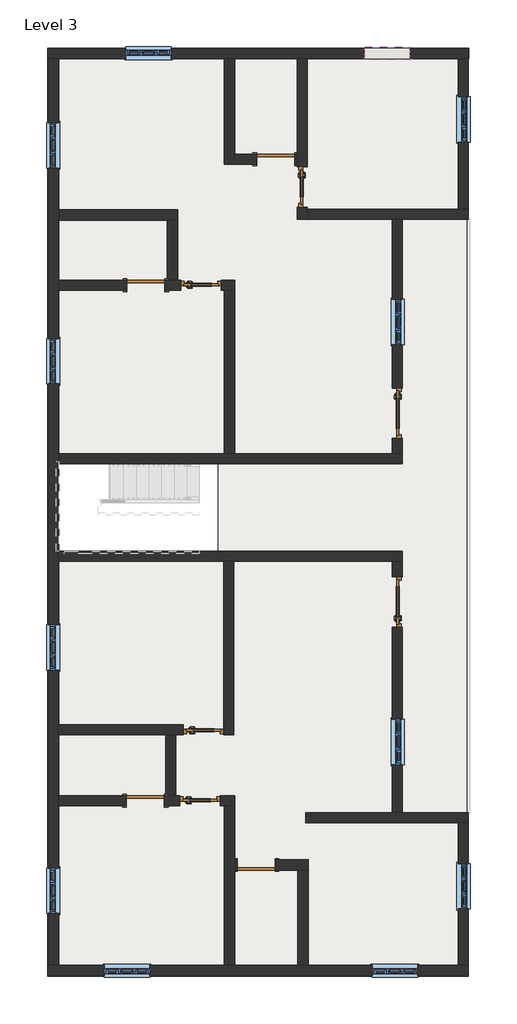
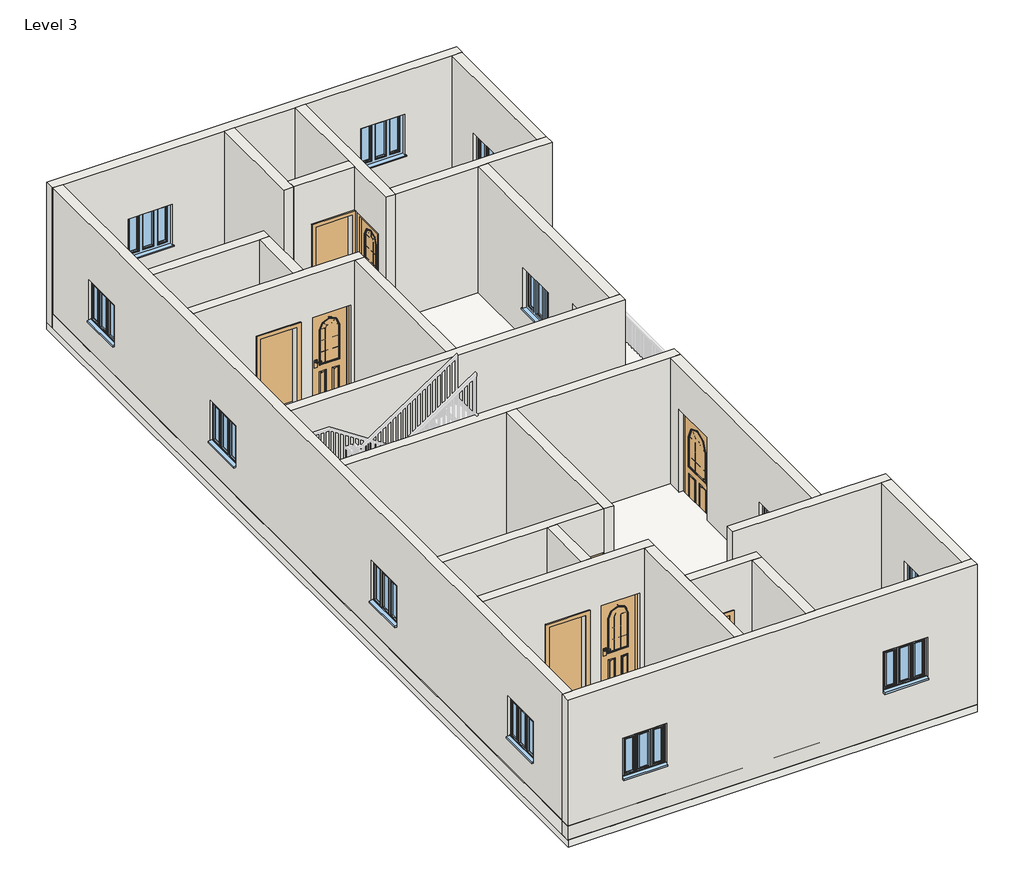
# One storey, part 1 of 3: 25 walls, 12 windows, 10 doors, 1 roof, 1 slab.
"""IFC4 building model written with IfcOpenShell, lengths in millimetres."""

from ifc_helpers import new_model, si_unit, frame, origin, place, context, project, spatial, polyline, outline, extrude, faceted_brep, transform, mapped, element, save
from components import doors_extsgl_w_glazing_bars_arched_1010x2110mm_bccdb1b2, doors_extsgl_w_glazing_bars_arched_1010x2110mm_5c897e1f, doors_extsgl_w_glazing_bars_arched_810x2110mm_57ea6d9e, doors_extsgl_w_glazing_bars_arched_810x2110mm_84a0a083, door_fadea3f2, windows_tpl_w_glazing_bars_910x910mm_9d987a72

model = new_model("IFC4")

# Units and contexts
model_context = context("Model", 3, world=origin())
ifc_project = project(units=[si_unit("LENGTHUNIT", "METRE", prefix="MILLI")], contexts=[model_context])

# Site, building, storey
site = spatial("IfcSite", under=ifc_project)
building = spatial("IfcBuilding", under=site)
storey = spatial("IfcBuildingStorey", under=building, Name="Level 3", Elevation=6096.0)

# Doors
placement = place(None, origin())
doors_extsgl_w_glazing_bars_arched_1010x2110mm_shape = doors_extsgl_w_glazing_bars_arched_1010x2110mm_bccdb1b2(model_context)
element("IfcDoor", 1, ObjectType="Doors_ExtSgl_w-Glazing_Bars_Arched : 1010x2110mm", at=placement, inside=storey, context=model_context, shape_type="MappedRepresentation", body=[
    mapped(doors_extsgl_w_glazing_bars_arched_1010x2110mm_shape, transform((1850.5605895, 2208.5797121, 6096.0), x_axis=(0.0, -1.0, 0.0), y_axis=(1.0, 0.0, 0.0), z_axis=(0.0, 0.0, 1.0))),
])
doors_extsgl_w_glazing_bars_arched_1010x2110mm_2_shape = doors_extsgl_w_glazing_bars_arched_1010x2110mm_5c897e1f(model_context)
element("IfcDoor", 2, ObjectType="Doors_ExtSgl_w-Glazing_Bars_Arched : 1010x2110mm", at=placement, inside=storey, context=model_context, shape_type="MappedRepresentation", body=[
    mapped(doors_extsgl_w_glazing_bars_arched_1010x2110mm_2_shape, transform((1850.5605895, -1576.0202879, 6096.0), x_axis=(0.0, 1.0, 0.0), y_axis=(-1.0, 0.0, 0.0), z_axis=(0.0, 0.0, 1.0))),
])
doors_extsgl_w_glazing_bars_arched_810x2110mm_shape = doors_extsgl_w_glazing_bars_arched_810x2110mm_57ea6d9e(model_context)
element("IfcDoor", 3, ObjectType="Doors_ExtSgl_w-Glazing_Bars_Arched : 810x2110mm", at=placement, inside=storey, context=model_context, shape_type="MappedRepresentation", body=[
    mapped(doors_extsgl_w_glazing_bars_arched_810x2110mm_shape, transform((-2086.4394105, 4773.9797121, 6096.0), x_axis=(1.0, 0.0, 0.0), y_axis=(0.0, 1.0, 0.0), z_axis=(0.0, 0.0, 1.0))),
])
element("IfcDoor", 4, ObjectType="Doors_ExtSgl_w-Glazing_Bars_Arched : 810x2110mm", at=placement, inside=storey, context=model_context, shape_type="MappedRepresentation", body=[
    mapped(doors_extsgl_w_glazing_bars_arched_810x2110mm_shape, transform((-2105.4894105, -5563.8202879, 6096.0), x_axis=(1.0, 0.0, 0.0), y_axis=(0.0, 1.0, 0.0), z_axis=(0.0, 0.0, 1.0))),
])
doors_extsgl_w_glazing_bars_arched_810x2110mm_2_shape = doors_extsgl_w_glazing_bars_arched_810x2110mm_84a0a083(model_context)
element("IfcDoor", 5, ObjectType="Doors_ExtSgl_w-Glazing_Bars_Arched : 810x2110mm", at=placement, inside=storey, context=model_context, shape_type="MappedRepresentation", body=[
    mapped(doors_extsgl_w_glazing_bars_arched_810x2110mm_2_shape, transform((-2035.6394105, -4141.4202879, 6096.0), x_axis=(1.0, 0.0, 0.0), y_axis=(0.0, 1.0, 0.0), z_axis=(0.0, 0.0, 1.0))),
])
element("IfcDoor", 6, ObjectType="Doors_ExtSgl_w-Glazing_Bars_Arched : 810x2110mm", at=placement, inside=storey, context=model_context, shape_type="MappedRepresentation", body=[
    mapped(doors_extsgl_w_glazing_bars_arched_810x2110mm_2_shape, transform((-54.4394105, 6748.5640518, 6096.0), x_axis=(0.0, -1.0, 0.0), y_axis=(1.0, 0.0, 0.0), z_axis=(0.0, 0.0, 1.0))),
])
door_shape = door_fadea3f2(model_context)
element("IfcDoor", 7, ObjectType="Single-Flush : 30\" x 80\"", at=placement, inside=storey, context=model_context, shape_type="MappedRepresentation", body=[
    mapped(door_shape, transform((-3204.0394105, -5563.8202879, 6096.0), x_axis=(1.0, 0.0, 0.0), y_axis=(0.0, 1.0, 0.0), z_axis=(0.0, 0.0, 1.0))),
])
element("IfcDoor", 8, ObjectType="Single-Flush : 30\" x 80\"", at=placement, inside=storey, context=model_context, shape_type="MappedRepresentation", body=[
    mapped(door_shape, transform((-981.5394105, -6850.9128362, 6096.0), x_axis=(-1.0, 0.0, 0.0), y_axis=(0.0, -1.0, 0.0), z_axis=(0.0, 0.0, 1.0))),
])
element("IfcDoor", 9, ObjectType="Single-Flush : 30\" x 80\"", at=placement, inside=storey, context=model_context, shape_type="MappedRepresentation", body=[
    mapped(door_shape, transform((-3191.3394105, 4773.9797121, 6096.0), x_axis=(1.0, 0.0, 0.0), y_axis=(0.0, 1.0, 0.0), z_axis=(0.0, 0.0, 1.0))),
])
element("IfcDoor", 10, ObjectType="Single-Flush : 30\" x 80\"", at=placement, inside=storey, context=model_context, shape_type="MappedRepresentation", body=[
    mapped(door_shape, transform((-587.8394105, 7301.2797121, 6096.0), x_axis=(1.0, 0.0, 0.0), y_axis=(0.0, 1.0, 0.0), z_axis=(0.0, 0.0, 1.0))),
])

# Roof
element("IfcRoof", 11, ObjectType="Generic - 12\"", at=placement, inside=storey, context=model_context, shape_type="SweptSolid", body=[
    extrude(outline(polyline([(3272.9605895, 9523.7797121), (3272.9605895, -9069.0202879), (-5159.8394105, -9069.0202879), (-5159.8394105, 9523.7797121), (3272.9605895, 9523.7797121)]), holes=[polyline([(-1756.1922756, 1192.5797121), (-4943.9394105, 1192.5797121), (-4943.9394105, -560.0202879), (-1756.1922756, -560.0202879), (-1756.1922756, 1192.5797121)])]), frame((0.0, 0.0, 6096.0), z_axis=(0.0, 0.0, 1.0), x_axis=(1.0, 0.0, 0.0)), (0.0, 0.0, 1.0), 304.8),
])

# Slab
element("IfcSlab", 12, ObjectType="Generic - 12\"", at=placement, inside=storey, context=model_context, shape_type="SweptSolid", body=[
    extrude(outline(polyline([(3272.9605895, 9523.7797121), (3272.9605895, -9081.7202879), (-5159.8394105, -9081.7202879), (-5159.8394105, 9523.7797121), (3272.9605895, 9523.7797121)]), holes=[polyline([(-1756.1922756, 1192.5797121), (-4943.9394105, 1192.5797121), (-4943.9394105, -560.0202879), (-1756.1922756, -560.0202879), (-1756.1922756, 1192.5797121)])]), frame((0.0, 0.0, 5943.6), z_axis=(0.0, 0.0, 1.0), x_axis=(1.0, 0.0, 0.0)), (0.0, 0.0, 1.0), 152.4),
])

# Walls
element("IfcWall", 13, ObjectType="Generic - 4.5\" p", at=placement, inside=storey, context=model_context, shape_type="Brep", body=[
    faceted_brep([(-2810.3394105, 4672.3797121, 8128.0), (-2810.3394105, 4672.3797121, 6096.0), (-2491.4394105, 4672.3797121, 6096.0), (-2491.4394105, 4672.3797121, 8206.0), (-1681.4394105, 4672.3797121, 8206.0), (-1681.4394105, 4672.3797121, 6096.0), (-1616.5394105, 4672.3797121, 6096.0), (-1413.3394105, 4672.3797121, 6096.0), (-1413.3394105, 4672.3797121, 9144.0), (-1616.5394105, 4672.3797121, 9144.0), (-4943.9394105, 4672.3797121, 9144.0), (-4943.9394105, 4672.3797121, 6096.0), (-3572.3394105, 4672.3797121, 6096.0), (-3572.3394105, 4672.3797121, 8128.0), (-2491.4394105, 4875.5797121, 6096.0), (-2556.3394105, 4875.5797121, 6096.0), (-2759.5394105, 4875.5797121, 6096.0), (-2810.3394105, 4875.5797121, 6096.0), (-2810.3394105, 4875.5797121, 8128.0), (-3572.3394105, 4875.5797121, 8128.0), (-3572.3394105, 4875.5797121, 6096.0), (-4943.9394105, 4875.5797121, 6096.0), (-4943.9394105, 4875.5797121, 9144.0), (-2759.5394105, 4875.5797121, 9144.0), (-2556.3394105, 4875.5797121, 9144.0), (-1413.3394105, 4875.5797121, 9144.0), (-1413.3394105, 4875.5797121, 6096.0), (-1681.4394105, 4875.5797121, 6096.0), (-1681.4394105, 4875.5797121, 8206.0), (-2491.4394105, 4875.5797121, 8206.0)], [[[0, 1, 2, 3, 4, 5, 6, 7, 8, 9, 10, 11, 12, 13]], [[14, 15, 16, 17, 18, 19, 20, 21, 22, 23, 24, 25, 26, 27, 28, 29]], [[7, 6, 5, 27, 26]], [[12, 11, 21, 20]], [[2, 1, 17, 16, 15, 14]], [[10, 9, 8, 25, 24, 23, 22]], [[11, 10, 22, 21]], [[8, 7, 26, 25]], [[14, 29, 3, 2]], [[28, 27, 5, 4]], [[29, 28, 4, 3]], [[18, 17, 1, 0]], [[19, 18, 0, 13]], [[20, 19, 13, 12]]]),
])
element("IfcWall", 14, ObjectType="Generic - 4.5\" p", at=placement, inside=storey, context=model_context, shape_type="SweptSolid", body=[
    extrude(outline(polyline([(-1616.5394105, 1395.7797121), (-1616.5394105, 4672.3797121), (-1413.3394105, 4672.3797121), (-1413.3394105, 1395.7797121), (-1616.5394105, 1395.7797121)])), frame((0.0, 0.0, 6096.0), z_axis=(0.0, 0.0, 1.0), x_axis=(1.0, 0.0, 0.0)), (0.0, 0.0, 1.0), 3048.0),
])
element("IfcWall", 15, ObjectType="Generic - 4.5\" p", at=placement, inside=storey, context=model_context, shape_type="Brep", body=[
    faceted_brep([(-4943.9394105, 6082.1542467, 6096.0), (-2759.5394105, 6082.1542467, 6096.0), (-2556.3394105, 6082.1542467, 6096.0), (-2556.3394105, 6082.1542467, 9144.0), (-2759.5394105, 6082.1542467, 9144.0), (-4943.9394105, 6082.1542467, 9144.0), (-4943.9394105, 6285.3542467, 6096.0), (-4943.9394105, 6285.3542467, 9144.0), (-2556.3394105, 6285.3542467, 9144.0), (-2556.3394105, 6285.3542467, 6096.0)], [[[0, 1, 2, 3, 4, 5]], [[6, 7, 8, 9]], [[2, 1, 0, 6, 9]], [[5, 4, 3, 8, 7]], [[0, 5, 7, 6]], [[3, 2, 9, 8]]]),
])
element("IfcWall", 16, ObjectType="Generic - 4.5\" p", at=placement, inside=storey, context=model_context, shape_type="SweptSolid", body=[
    extrude(outline(polyline([(-2759.5394105, 4875.5797121), (-2759.5394105, 6082.1542467), (-2556.3394105, 6082.1542467), (-2556.3394105, 4875.5797121), (-2759.5394105, 4875.5797121)])), frame((0.0, 0.0, 6096.0), z_axis=(0.0, 0.0, 1.0), x_axis=(1.0, 0.0, 0.0)), (0.0, 0.0, 1.0), 3048.0),
])
element("IfcWall", 17, ObjectType="Generic - 4.5\" p", at=placement, inside=storey, context=model_context, shape_type="Brep", body=[
    faceted_brep([(-1616.5394105, 9320.5797121, 6096.0), (-1616.5394105, 7199.6797121, 6096.0), (-1616.5394105, 7199.6797121, 9144.0), (-1616.5394105, 9320.5797121, 9144.0), (-1413.3394105, 9320.5797121, 6096.0), (-1413.3394105, 9320.5797121, 9144.0), (-1413.3394105, 7402.8797121, 9144.0), (-1413.3394105, 7199.6797121, 9144.0), (-1413.3394105, 7199.6797121, 6096.0), (-1413.3394105, 7402.8797121, 6096.0)], [[[0, 1, 2, 3]], [[4, 5, 6, 7, 8, 9]], [[1, 0, 4, 9, 8]], [[3, 2, 7, 6, 5]], [[0, 3, 5, 4]], [[2, 1, 8, 7]]]),
])
element("IfcWall", 18, ObjectType="Generic - 4.5\" p", at=placement, inside=storey, context=model_context, shape_type="SweptSolid", body=[
    extrude(outline(polyline([(8128.0, -206.8394105), (6096.0, -206.8394105), (6096.0, -156.0394105), (9144.0, -156.0394105), (9144.0, -1413.3394105), (6096.0, -1413.3394105), (6096.0, -968.8394105), (8128.0, -968.8394105), (8128.0, -206.8394105)])), frame((0.0, 7199.6797121, 0.0), z_axis=(0.0, 1.0, 0.0), x_axis=(0.0, 0.0, 1.0)), (0.0, 0.0, 1.0), 203.2),
])
element("IfcWall", 19, ObjectType="Generic - 4.5\" p", at=placement, inside=storey, context=model_context, shape_type="Brep", body=[
    faceted_brep([(-156.0394105, 6343.5640518, 8206.0), (-156.0394105, 6343.5640518, 6096.0), (-156.0394105, 6094.2483916, 6096.0), (-156.0394105, 6094.2483916, 9144.0), (-156.0394105, 7199.6797121, 9144.0), (-156.0394105, 7402.8797121, 9144.0), (-156.0394105, 9320.5797121, 9144.0), (-156.0394105, 9320.5797121, 6096.0), (-156.0394105, 7402.8797121, 6096.0), (-156.0394105, 7199.6797121, 6096.0), (-156.0394105, 7153.5640518, 6096.0), (-156.0394105, 7153.5640518, 8206.0), (47.1605895, 6094.2483916, 6096.0), (47.1605895, 6297.4483916, 6096.0), (47.1605895, 6343.5640518, 6096.0), (47.1605895, 6343.5640518, 8206.0), (47.1605895, 7153.5640518, 8206.0), (47.1605895, 7153.5640518, 6096.0), (47.1605895, 9320.5797121, 6096.0), (47.1605895, 9320.5797121, 9144.0), (47.1605895, 6297.4483916, 9144.0), (47.1605895, 6094.2483916, 9144.0)], [[[0, 1, 2, 3, 4, 5, 6, 7, 8, 9, 10, 11]], [[12, 13, 14, 15, 16, 17, 18, 19, 20, 21]], [[2, 1, 14, 13, 12]], [[10, 9, 8, 7, 18, 17]], [[6, 5, 4, 3, 21, 20, 19]], [[7, 6, 19, 18]], [[3, 2, 12, 21]], [[17, 16, 11, 10]], [[15, 14, 1, 0]], [[16, 15, 0, 11]]]),
])
element("IfcWall", 20, ObjectType="Generic - 4.5\" p", at=placement, inside=storey, context=model_context, shape_type="Brep", body=[
    faceted_brep([(47.1605895, 6094.2483916, 6096.0), (1748.9605895, 6094.2483916, 6096.0), (1952.1605895, 6094.2483916, 6096.0), (3272.9605895, 6094.2483916, 6096.0), (3272.9605895, 6094.2483916, 9144.0), (1952.1605895, 6094.2483916, 9144.0), (1748.9605895, 6094.2483916, 9144.0), (47.1605895, 6094.2483916, 9144.0), (47.1605895, 6297.4483916, 6096.0), (47.1605895, 6297.4483916, 9144.0), (3069.7605895, 6297.4483916, 9144.0), (3272.9605895, 6297.4483916, 9144.0), (3272.9605895, 6297.4483916, 6096.0), (3069.7605895, 6297.4483916, 6096.0)], [[[0, 1, 2, 3, 4, 5, 6, 7]], [[8, 9, 10, 11, 12, 13]], [[3, 2, 1, 0, 8, 13, 12]], [[7, 6, 5, 4, 11, 10, 9]], [[0, 7, 9, 8]], [[4, 3, 12, 11]]]),
])
element("IfcWall", 21, ObjectType="Generic - 4.5\" p", at=placement, inside=storey, context=model_context, shape_type="Brep", body=[
    faceted_brep([(-4943.9394105, 1192.5797121, 6096.0), (1952.1605895, 1192.5797121, 6096.0), (1952.1605895, 1192.5797121, 9144.0), (-4943.9394105, 1192.5797121, 9144.0), (-4943.9394105, 1395.7797121, 6096.0), (-4943.9394105, 1395.7797121, 9144.0), (-1616.5394105, 1395.7797121, 9144.0), (-1413.3394105, 1395.7797121, 9144.0), (1748.9605895, 1395.7797121, 9144.0), (1952.1605895, 1395.7797121, 9144.0), (1952.1605895, 1395.7797121, 6096.0), (1748.9605895, 1395.7797121, 6096.0), (-1413.3394105, 1395.7797121, 6096.0), (-1616.5394105, 1395.7797121, 6096.0)], [[[0, 1, 2, 3]], [[4, 5, 6, 7, 8, 9, 10, 11, 12, 13]], [[1, 0, 4, 13, 12, 11, 10]], [[3, 2, 9, 8, 7, 6, 5]], [[0, 3, 5, 4]], [[2, 1, 10, 9]]]),
])
element("IfcWall", 22, ObjectType="Generic - 4.5\" p", at=placement, inside=storey, context=model_context, shape_type="Brep", body=[
    faceted_brep([(-4943.9394105, -763.2202879, 6096.0), (-1629.2394105, -763.2202879, 6096.0), (-1426.0394105, -763.2202879, 6096.0), (1748.9605895, -763.2202879, 6096.0), (1952.1605895, -763.2202879, 6096.0), (1952.1605895, -763.2202879, 9144.0), (1748.9605895, -763.2202879, 9144.0), (-1426.0394105, -763.2202879, 9144.0), (-1629.2394105, -763.2202879, 9144.0), (-4943.9394105, -763.2202879, 9144.0), (-4943.9394105, -560.0202879, 6096.0), (-4943.9394105, -560.0202879, 9144.0), (1952.1605895, -560.0202879, 9144.0), (1952.1605895, -560.0202879, 6096.0)], [[[0, 1, 2, 3, 4, 5, 6, 7, 8, 9]], [[10, 11, 12, 13]], [[4, 3, 2, 1, 0, 10, 13]], [[9, 8, 7, 6, 5, 12, 11]], [[0, 9, 11, 10]], [[5, 4, 13, 12]]]),
])
element("IfcWall", 23, ObjectType="Generic - 4.5\" p", at=placement, inside=storey, context=model_context, shape_type="Brep", body=[
    faceted_brep([(-1629.2394105, -763.2202879, 6096.0), (-1629.2394105, -4039.8202879, 6096.0), (-1629.2394105, -4243.0202879, 6096.0), (-1629.2394105, -4243.0202879, 9144.0), (-1629.2394105, -4039.8202879, 9144.0), (-1629.2394105, -763.2202879, 9144.0), (-1426.0394105, -763.2202879, 6096.0), (-1426.0394105, -763.2202879, 9144.0), (-1426.0394105, -4243.0202879, 9144.0), (-1426.0394105, -4243.0202879, 6096.0)], [[[0, 1, 2, 3, 4, 5]], [[6, 7, 8, 9]], [[2, 1, 0, 6, 9]], [[5, 4, 3, 8, 7]], [[0, 5, 7, 6]], [[3, 2, 9, 8]]]),
])
element("IfcWall", 24, ObjectType="Generic - 4.5\" p", at=placement, inside=storey, context=model_context, shape_type="Brep", body=[
    faceted_brep([(-1630.6394105, -4243.0202879, 8206.0), (-1630.6394105, -4243.0202879, 6096.0), (-1629.2394105, -4243.0202879, 6096.0), (-1629.2394105, -4243.0202879, 9144.0), (-2594.4394105, -4243.0202879, 9144.0), (-2797.6394105, -4243.0202879, 9144.0), (-4943.9394105, -4243.0202879, 9144.0), (-4943.9394105, -4243.0202879, 6096.0), (-2797.6394105, -4243.0202879, 6096.0), (-2594.4394105, -4243.0202879, 6096.0), (-2440.6394105, -4243.0202879, 6096.0), (-2440.6394105, -4243.0202879, 8206.0), (-1629.2394105, -4039.8202879, 6096.0), (-1630.6394105, -4039.8202879, 6096.0), (-1630.6394105, -4039.8202879, 8206.0), (-2440.6394105, -4039.8202879, 8206.0), (-2440.6394105, -4039.8202879, 6096.0), (-4943.9394105, -4039.8202879, 6096.0), (-4943.9394105, -4039.8202879, 9144.0), (-1629.2394105, -4039.8202879, 9144.0)], [[[0, 1, 2, 3, 4, 5, 6, 7, 8, 9, 10, 11]], [[12, 13, 14, 15, 16, 17, 18, 19]], [[2, 1, 13, 12]], [[10, 9, 8, 7, 17, 16]], [[6, 5, 4, 3, 19, 18]], [[3, 2, 12, 19]], [[7, 6, 18, 17]], [[16, 15, 11, 10]], [[14, 13, 1, 0]], [[15, 14, 0, 11]]]),
])
element("IfcWall", 25, ObjectType="Generic - 4.5\" p", at=placement, inside=storey, context=model_context, shape_type="Brep", body=[
    faceted_brep([(-2823.0394105, -5665.4202879, 8128.0), (-2823.0394105, -5665.4202879, 6096.0), (-2510.4894105, -5665.4202879, 6096.0), (-2510.4894105, -5665.4202879, 8206.0), (-1700.4894105, -5665.4202879, 8206.0), (-1700.4894105, -5665.4202879, 6096.0), (-1616.5394105, -5665.4202879, 6096.0), (-1413.3394105, -5665.4202879, 6096.0), (-1413.3394105, -5665.4202879, 9144.0), (-1616.5394105, -5665.4202879, 9144.0), (-4943.9394105, -5665.4202879, 9144.0), (-4943.9394105, -5665.4202879, 6096.0), (-3585.0394105, -5665.4202879, 6096.0), (-3585.0394105, -5665.4202879, 8128.0), (-2510.4894105, -5462.2202879, 6096.0), (-2594.4394105, -5462.2202879, 6096.0), (-2797.6394105, -5462.2202879, 6096.0), (-2823.0394105, -5462.2202879, 6096.0), (-2823.0394105, -5462.2202879, 8128.0), (-3585.0394105, -5462.2202879, 8128.0), (-3585.0394105, -5462.2202879, 6096.0), (-4943.9394105, -5462.2202879, 6096.0), (-4943.9394105, -5462.2202879, 9144.0), (-2797.6394105, -5462.2202879, 9144.0), (-2594.4394105, -5462.2202879, 9144.0), (-1413.3394105, -5462.2202879, 9144.0), (-1413.3394105, -5462.2202879, 6096.0), (-1700.4894105, -5462.2202879, 6096.0), (-1700.4894105, -5462.2202879, 8206.0), (-2510.4894105, -5462.2202879, 8206.0)], [[[0, 1, 2, 3, 4, 5, 6, 7, 8, 9, 10, 11, 12, 13]], [[14, 15, 16, 17, 18, 19, 20, 21, 22, 23, 24, 25, 26, 27, 28, 29]], [[7, 6, 5, 27, 26]], [[12, 11, 21, 20]], [[2, 1, 17, 16, 15, 14]], [[10, 9, 8, 25, 24, 23, 22]], [[11, 10, 22, 21]], [[8, 7, 26, 25]], [[14, 29, 3, 2]], [[28, 27, 5, 4]], [[29, 28, 4, 3]], [[18, 17, 1, 0]], [[19, 18, 0, 13]], [[20, 19, 13, 12]]]),
])
element("IfcWall", 26, ObjectType="Generic - 4.5\" p", at=placement, inside=storey, context=model_context, shape_type="SweptSolid", body=[
    extrude(outline(polyline([(-2797.6394105, -5462.2202879), (-2797.6394105, -4243.0202879), (-2594.4394105, -4243.0202879), (-2594.4394105, -5462.2202879), (-2797.6394105, -5462.2202879)])), frame((0.0, 0.0, 6096.0), z_axis=(0.0, 0.0, 1.0), x_axis=(1.0, 0.0, 0.0)), (0.0, 0.0, 1.0), 3048.0),
])
element("IfcWall", 27, ObjectType="Generic - 4.5\" p", at=placement, inside=storey, context=model_context, shape_type="Brep", body=[
    faceted_brep([(-1616.5394105, -5665.4202879, 6096.0), (-1616.5394105, -8865.8202879, 6096.0), (-1616.5394105, -8865.8202879, 9144.0), (-1616.5394105, -5665.4202879, 9144.0), (-1413.3394105, -5665.4202879, 6096.0), (-1413.3394105, -5665.4202879, 9144.0), (-1413.3394105, -6749.3128362, 9144.0), (-1413.3394105, -6952.5128362, 9144.0), (-1413.3394105, -8865.8202879, 9144.0), (-1413.3394105, -8865.8202879, 6096.0), (-1413.3394105, -6952.5128362, 6096.0), (-1413.3394105, -6749.3128362, 6096.0)], [[[0, 1, 2, 3]], [[4, 5, 6, 7, 8, 9, 10, 11]], [[1, 0, 4, 11, 10, 9]], [[3, 2, 8, 7, 6, 5]], [[0, 3, 5, 4]], [[2, 1, 9, 8]]]),
])
element("IfcWall", 28, ObjectType="Generic - 4.5\" p", at=placement, inside=storey, context=model_context, shape_type="Brep", body=[
    faceted_brep([(-1413.3394105, -6952.5128362, 6096.0), (-1362.5394105, -6952.5128362, 6096.0), (-1362.5394105, -6952.5128362, 8128.0), (-600.5394105, -6952.5128362, 8128.0), (-600.5394105, -6952.5128362, 6096.0), (-143.3394105, -6952.5128362, 6096.0), (59.8605895, -6952.5128362, 6096.0), (59.8605895, -6952.5128362, 9144.0), (-143.3394105, -6952.5128362, 9144.0), (-1413.3394105, -6952.5128362, 9144.0), (-1362.5394105, -6749.3128362, 8128.0), (-1362.5394105, -6749.3128362, 6096.0), (-1413.3394105, -6749.3128362, 6096.0), (-1413.3394105, -6749.3128362, 9144.0), (59.8605895, -6749.3128362, 9144.0), (59.8605895, -6749.3128362, 6096.0), (-600.5394105, -6749.3128362, 6096.0), (-600.5394105, -6749.3128362, 8128.0)], [[[0, 1, 2, 3, 4, 5, 6, 7, 8, 9]], [[10, 11, 12, 13, 14, 15, 16, 17]], [[16, 15, 6, 5, 4]], [[12, 11, 1, 0]], [[9, 8, 7, 14, 13]], [[0, 9, 13, 12]], [[7, 6, 15, 14]], [[2, 1, 11, 10]], [[3, 2, 10, 17]], [[4, 3, 17, 16]]]),
])
element("IfcWall", 29, ObjectType="Generic - 4.5\" p", at=placement, inside=storey, context=model_context, shape_type="SweptSolid", body=[
    extrude(outline(polyline([(-143.3394105, -8865.8202879), (-143.3394105, -6952.5128362), (59.8605895, -6952.5128362), (59.8605895, -8865.8202879), (-143.3394105, -8865.8202879)])), frame((0.0, 0.0, 6096.0), z_axis=(0.0, 0.0, 1.0), x_axis=(1.0, 0.0, 0.0)), (0.0, 0.0, 1.0), 3048.0),
])
element("IfcWall", 30, ObjectType="Generic - 4.5\" p", at=placement, inside=storey, context=model_context, shape_type="Brep", body=[
    faceted_brep([(3272.9605895, -5805.1202879, 6096.0), (1952.1605895, -5805.1202879, 6096.0), (1748.9605895, -5805.1202879, 6096.0), (9.0605895, -5805.1202879, 6096.0), (9.0605895, -5805.1202879, 9144.0), (1748.9605895, -5805.1202879, 9144.0), (1952.1605895, -5805.1202879, 9144.0), (3272.9605895, -5805.1202879, 9144.0), (3272.9605895, -6008.3202879, 6096.0), (3272.9605895, -6008.3202879, 9144.0), (3069.7605895, -6008.3202879, 9144.0), (9.0605895, -6008.3202879, 9144.0), (9.0605895, -6008.3202879, 6096.0), (3069.7605895, -6008.3202879, 6096.0)], [[[0, 1, 2, 3, 4, 5, 6, 7]], [[8, 9, 10, 11, 12, 13]], [[3, 2, 1, 0, 8, 13, 12]], [[4, 3, 12, 11]], [[7, 6, 5, 4, 11, 10, 9]], [[0, 7, 9, 8]]]),
])
element("IfcWall", 31, ObjectType="Generic - 9\" w", at=placement, inside=storey, context=model_context, shape_type="Brep", body=[
    faceted_brep([(-5159.8394105, 9320.5797121, 6096.0), (-5147.1394105, 9320.5797121, 6096.0), (-4943.9394105, 9320.5797121, 6096.0), (-1616.5394105, 9320.5797121, 6096.0), (-1413.3394105, 9320.5797121, 6096.0), (-156.0394105, 9320.5797121, 6096.0), (47.1605895, 9320.5797121, 6096.0), (3069.7605895, 9320.5797121, 6096.0), (3272.9605895, 9320.5797121, 6096.0), (3285.6605895, 9320.5797121, 6096.0), (3285.6605895, 9320.5797121, 9144.0), (3272.9605895, 9320.5797121, 9144.0), (3069.7605895, 9320.5797121, 9144.0), (47.1605895, 9320.5797121, 9144.0), (-156.0394105, 9320.5797121, 9144.0), (-1413.3394105, 9320.5797121, 9144.0), (-1616.5394105, 9320.5797121, 9144.0), (-4943.9394105, 9320.5797121, 9144.0), (-5147.1394105, 9320.5797121, 9144.0), (-5159.8394105, 9320.5797121, 9144.0), (1192.3605895, 9320.5797121, 8206.0), (2102.3605895, 9320.5797121, 8206.0), (2102.3605895, 9320.5797121, 7296.0), (1192.3605895, 9320.5797121, 7296.0), (-3595.5394105, 9320.5797121, 7920.4), (-2685.5394105, 9320.5797121, 7920.4), (-2685.5394105, 9320.5797121, 7010.4), (-3595.5394105, 9320.5797121, 7010.4), (-5159.8394105, 9523.7797121, 6096.0), (-5159.8394105, 9523.7797121, 9144.0), (3285.6605895, 9523.7797121, 9144.0), (3285.6605895, 9523.7797121, 6096.0), (1192.3605895, 9523.7797121, 8206.0), (1192.3605895, 9523.7797121, 7296.0), (2102.3605895, 9523.7797121, 7296.0), (2102.3605895, 9523.7797121, 8206.0), (-3595.5394105, 9523.7797121, 7920.4), (-3595.5394105, 9523.7797121, 7010.4), (-2685.5394105, 9523.7797121, 7010.4), (-2685.5394105, 9523.7797121, 7920.4)], [[[0, 1, 2, 3, 4, 5, 6, 7, 8, 9, 10, 11, 12, 13, 14, 15, 16, 17, 18, 19], [20, 21, 22, 23], [24, 25, 26, 27]], [[28, 29, 30, 31], [32, 33, 34, 35], [36, 37, 38, 39]], [[9, 8, 7, 6, 5, 4, 3, 2, 1, 0, 28, 31]], [[10, 9, 31, 30]], [[19, 18, 17, 16, 15, 14, 13, 12, 11, 10, 30, 29]], [[0, 19, 29, 28]], [[33, 32, 20, 23]], [[34, 33, 23, 22]], [[35, 34, 22, 21]], [[32, 35, 21, 20]], [[37, 36, 24, 27]], [[38, 37, 27, 26]], [[39, 38, 26, 25]], [[36, 39, 25, 24]]]),
])
element("IfcWall", 32, ObjectType="Generic - 9\" w", at=placement, inside=storey, context=model_context, shape_type="Brep", body=[
    faceted_brep([(3272.9605895, -8865.8202879, 6096.0), (3069.7605895, -8865.8202879, 6096.0), (59.8605895, -8865.8202879, 6096.0), (-143.3394105, -8865.8202879, 6096.0), (-1413.3394105, -8865.8202879, 6096.0), (-1616.5394105, -8865.8202879, 6096.0), (-4943.9394105, -8865.8202879, 6096.0), (-5147.1394105, -8865.8202879, 6096.0), (-5159.8394105, -8865.8202879, 6096.0), (-5159.8394105, -8865.8202879, 9144.0), (-5147.1394105, -8865.8202879, 9144.0), (-4943.9394105, -8865.8202879, 9144.0), (-1616.5394105, -8865.8202879, 9144.0), (-1413.3394105, -8865.8202879, 9144.0), (-143.3394105, -8865.8202879, 9144.0), (59.8605895, -8865.8202879, 9144.0), (3069.7605895, -8865.8202879, 9144.0), (3272.9605895, -8865.8202879, 9144.0), (-3117.3394105, -8865.8202879, 7920.4), (-4027.3394105, -8865.8202879, 7920.4), (-4027.3394105, -8865.8202879, 7010.4), (-3117.3394105, -8865.8202879, 7010.4), (2254.7605895, -8865.8202879, 7920.4), (1344.7605895, -8865.8202879, 7920.4), (1344.7605895, -8865.8202879, 7010.4), (2254.7605895, -8865.8202879, 7010.4), (3272.9605895, -9069.0202879, 6096.0), (3272.9605895, -9069.0202879, 9144.0), (-5159.8394105, -9069.0202879, 9144.0), (-5159.8394105, -9069.0202879, 6096.0), (-3117.3394105, -9069.0202879, 7920.4), (-3117.3394105, -9069.0202879, 7010.4), (-4027.3394105, -9069.0202879, 7010.4), (-4027.3394105, -9069.0202879, 7920.4), (2254.7605895, -9069.0202879, 7920.4), (2254.7605895, -9069.0202879, 7010.4), (1344.7605895, -9069.0202879, 7010.4), (1344.7605895, -9069.0202879, 7920.4)], [[[0, 1, 2, 3, 4, 5, 6, 7, 8, 9, 10, 11, 12, 13, 14, 15, 16, 17], [18, 19, 20, 21], [22, 23, 24, 25]], [[26, 27, 28, 29], [30, 31, 32, 33], [34, 35, 36, 37]], [[8, 7, 6, 5, 4, 3, 2, 1, 0, 26, 29]], [[9, 8, 29, 28]], [[17, 16, 15, 14, 13, 12, 11, 10, 9, 28, 27]], [[0, 17, 27, 26]], [[31, 30, 18, 21]], [[32, 31, 21, 20]], [[33, 32, 20, 19]], [[30, 33, 19, 18]], [[35, 34, 22, 25]], [[36, 35, 25, 24]], [[37, 36, 24, 23]], [[34, 37, 23, 22]]]),
])
element("IfcWall", 33, ObjectType="Generic - 9\" w", at=placement, inside=storey, context=model_context, shape_type="Brep", body=[
    faceted_brep([(-4943.9394105, -8865.8202879, 6096.0), (-4943.9394105, -5665.4202879, 6096.0), (-4943.9394105, -5462.2202879, 6096.0), (-4943.9394105, -4243.0202879, 6096.0), (-4943.9394105, -4039.8202879, 6096.0), (-4943.9394105, -763.2202879, 6096.0), (-4943.9394105, -560.0202879, 6096.0), (-4943.9394105, 1192.5797121, 6096.0), (-4943.9394105, 1395.7797121, 6096.0), (-4943.9394105, 4672.3797121, 6096.0), (-4943.9394105, 4875.5797121, 6096.0), (-4943.9394105, 6082.1542467, 6096.0), (-4943.9394105, 6285.3542467, 6096.0), (-4943.9394105, 9320.5797121, 6096.0), (-4943.9394105, 9320.5797121, 9144.0), (-4943.9394105, 6285.3542467, 9144.0), (-4943.9394105, 6082.1542467, 9144.0), (-4943.9394105, 4875.5797121, 9144.0), (-4943.9394105, 4672.3797121, 9144.0), (-4943.9394105, 1395.7797121, 9144.0), (-4943.9394105, 1192.5797121, 9144.0), (-4943.9394105, -560.0202879, 9144.0), (-4943.9394105, -763.2202879, 9144.0), (-4943.9394105, -4039.8202879, 9144.0), (-4943.9394105, -4243.0202879, 9144.0), (-4943.9394105, -5462.2202879, 9144.0), (-4943.9394105, -5665.4202879, 9144.0), (-4943.9394105, -8865.8202879, 9144.0), (-4943.9394105, -7822.2202879, 7920.4), (-4943.9394105, -6912.2202879, 7920.4), (-4943.9394105, -6912.2202879, 7010.4), (-4943.9394105, -7822.2202879, 7010.4), (-4943.9394105, -2945.4202879, 7920.4), (-4943.9394105, -2035.4202879, 7920.4), (-4943.9394105, -2035.4202879, 7010.4), (-4943.9394105, -2945.4202879, 7010.4), (-4943.9394105, 2794.9797121, 7920.4), (-4943.9394105, 3704.9797121, 7920.4), (-4943.9394105, 3704.9797121, 7010.4), (-4943.9394105, 2794.9797121, 7010.4), (-4943.9394105, 7125.7542467, 7920.4), (-4943.9394105, 8035.7542467, 7920.4), (-4943.9394105, 8035.7542467, 7010.4), (-4943.9394105, 7125.7542467, 7010.4), (-5147.1394105, -8865.8202879, 6096.0), (-5147.1394105, -8865.8202879, 9144.0), (-5147.1394105, 9320.5797121, 9144.0), (-5147.1394105, 9320.5797121, 6096.0), (-5147.1394105, -7822.2202879, 7920.4), (-5147.1394105, -7822.2202879, 7010.4), (-5147.1394105, -6912.2202879, 7010.4), (-5147.1394105, -6912.2202879, 7920.4), (-5147.1394105, -2945.4202879, 7920.4), (-5147.1394105, -2945.4202879, 7010.4), (-5147.1394105, -2035.4202879, 7010.4), (-5147.1394105, -2035.4202879, 7920.4), (-5147.1394105, 2794.9797121, 7920.4), (-5147.1394105, 2794.9797121, 7010.4), (-5147.1394105, 3704.9797121, 7010.4), (-5147.1394105, 3704.9797121, 7920.4), (-5147.1394105, 7125.7542467, 7920.4), (-5147.1394105, 7125.7542467, 7010.4), (-5147.1394105, 8035.7542467, 7010.4), (-5147.1394105, 8035.7542467, 7920.4)], [[[0, 1, 2, 3, 4, 5, 6, 7, 8, 9, 10, 11, 12, 13, 14, 15, 16, 17, 18, 19, 20, 21, 22, 23, 24, 25, 26, 27], [28, 29, 30, 31], [32, 33, 34, 35], [36, 37, 38, 39], [40, 41, 42, 43]], [[44, 45, 46, 47], [48, 49, 50, 51], [52, 53, 54, 55], [56, 57, 58, 59], [60, 61, 62, 63]], [[13, 12, 11, 10, 9, 8, 7, 6, 5, 4, 3, 2, 1, 0, 44, 47]], [[27, 26, 25, 24, 23, 22, 21, 20, 19, 18, 17, 16, 15, 14, 46, 45]], [[14, 13, 47, 46]], [[0, 27, 45, 44]], [[49, 48, 28, 31]], [[50, 49, 31, 30]], [[51, 50, 30, 29]], [[48, 51, 29, 28]], [[53, 52, 32, 35]], [[54, 53, 35, 34]], [[55, 54, 34, 33]], [[52, 55, 33, 32]], [[57, 56, 36, 39]], [[58, 57, 39, 38]], [[59, 58, 38, 37]], [[56, 59, 37, 36]], [[61, 60, 40, 43]], [[62, 61, 43, 42]], [[63, 62, 42, 41]], [[60, 63, 41, 40]]]),
])
element("IfcWall", 34, ObjectType="Generic - 9\" w", at=placement, inside=storey, context=model_context, shape_type="SweptSolid", body=[
    extrude(outline(polyline([(-8865.8202879, 6096.0), (-8865.8202879, 9144.0), (-6008.3202879, 9144.0), (-6008.3202879, 6096.0), (-8865.8202879, 6096.0)]), holes=[polyline([(-6823.3202879, 7920.4), (-7733.3202879, 7920.4), (-7733.3202879, 7010.4), (-6823.3202879, 7010.4), (-6823.3202879, 7920.4)])]), frame((3069.7605895, 0.0, 0.0), z_axis=(1.0, 0.0, 0.0), x_axis=(0.0, 1.0, 0.0)), (0.0, 0.0, 1.0), 203.2),
])
element("IfcWall", 35, ObjectType="Generic - 9\" w", at=placement, inside=storey, context=model_context, shape_type="SweptSolid", body=[
    extrude(outline(polyline([(9320.5797121, 6096.0), (6297.4483916, 6096.0), (6297.4483916, 9144.0), (9320.5797121, 9144.0), (9320.5797121, 6096.0)]), holes=[polyline([(8556.3797121, 7920.4), (7646.3797121, 7920.4), (7646.3797121, 7010.4), (8556.3797121, 7010.4), (8556.3797121, 7920.4)])]), frame((3069.7605895, 0.0, 0.0), z_axis=(1.0, 0.0, 0.0), x_axis=(0.0, 1.0, 0.0)), (0.0, 0.0, 1.0), 203.2),
])
element("IfcWall", 36, ObjectType="Generic - 9\" w", at=placement, inside=storey, context=model_context, shape_type="SweptSolid", body=[
    extrude(outline(polyline([(-763.2202879, 6096.0), (-1071.0202879, 6096.0), (-1071.0202879, 8206.0), (-2081.0202879, 8206.0), (-2081.0202879, 6096.0), (-5805.1202879, 6096.0), (-5805.1202879, 9144.0), (-763.2202879, 9144.0), (-763.2202879, 6096.0)]), holes=[polyline([(-3927.7202879, 7920.4), (-4837.7202879, 7920.4), (-4837.7202879, 7010.4), (-3927.7202879, 7010.4), (-3927.7202879, 7920.4)])]), frame((1748.9605895, 0.0, 0.0), z_axis=(1.0, 0.0, 0.0), x_axis=(0.0, 1.0, 0.0)), (0.0, 0.0, 1.0), 203.2),
])
element("IfcWall", 37, ObjectType="Generic - 9\" w", at=placement, inside=storey, context=model_context, shape_type="SweptSolid", body=[
    extrude(outline(polyline([(1703.5797121, 8206.0), (1703.5797121, 6096.0), (1395.7797121, 6096.0), (1395.7797121, 9144.0), (6094.2483916, 9144.0), (6094.2483916, 6096.0), (2713.5797121, 6096.0), (2713.5797121, 8206.0), (1703.5797121, 8206.0)]), holes=[polyline([(4492.3797121, 7920.4), (3582.3797121, 7920.4), (3582.3797121, 7010.4), (4492.3797121, 7010.4), (4492.3797121, 7920.4)])]), frame((1748.9605895, 0.0, 0.0), z_axis=(1.0, 0.0, 0.0), x_axis=(0.0, 1.0, 0.0)), (0.0, 0.0, 1.0), 203.2),
])

# Windows
windows_tpl_w_glazing_bars_910x910mm_shape = windows_tpl_w_glazing_bars_910x910mm_9d987a72(model_context)
element("IfcWindow", 38, ObjectType="Windows_Tpl_w-Glazing_Bars : 910x910mm", at=placement, inside=storey, context=model_context, shape_type="MappedRepresentation", body=[
    mapped(windows_tpl_w_glazing_bars_910x910mm_shape, transform((-3809.0060772, -8958.9637201, 5810.4), x_axis=(-1.0, 0.0, 0.0), y_axis=(0.0, -1.0, 0.0), z_axis=(0.0, 0.0, 1.0))),
])
element("IfcWindow", 39, ObjectType="Windows_Tpl_w-Glazing_Bars : 910x910mm", at=placement, inside=storey, context=model_context, shape_type="MappedRepresentation", body=[
    mapped(windows_tpl_w_glazing_bars_910x910mm_shape, transform((-5037.0828427, -7130.5536213, 5810.4), x_axis=(0.0, 1.0, 0.0), y_axis=(-1.0, 0.0, 0.0), z_axis=(0.0, 0.0, 1.0))),
])
element("IfcWindow", 40, ObjectType="Windows_Tpl_w-Glazing_Bars : 910x910mm", at=placement, inside=storey, context=model_context, shape_type="MappedRepresentation", body=[
    mapped(windows_tpl_w_glazing_bars_910x910mm_shape, transform((-5037.0828427, -2253.7536213, 5810.4), x_axis=(0.0, 1.0, 0.0), y_axis=(-1.0, 0.0, 0.0), z_axis=(0.0, 0.0, 1.0))),
])
element("IfcWindow", 41, ObjectType="Windows_Tpl_w-Glazing_Bars : 910x910mm", at=placement, inside=storey, context=model_context, shape_type="MappedRepresentation", body=[
    mapped(windows_tpl_w_glazing_bars_910x910mm_shape, transform((-5037.0828427, 3486.6463787, 5810.4), x_axis=(0.0, 1.0, 0.0), y_axis=(-1.0, 0.0, 0.0), z_axis=(0.0, 0.0, 1.0))),
])
element("IfcWindow", 42, ObjectType="Windows_Tpl_w-Glazing_Bars : 910x910mm", at=placement, inside=storey, context=model_context, shape_type="MappedRepresentation", body=[
    mapped(windows_tpl_w_glazing_bars_910x910mm_shape, transform((3162.9040216, 7864.7130454, 5810.4), x_axis=(0.0, -1.0, 0.0), y_axis=(1.0, 0.0, 0.0), z_axis=(0.0, 0.0, 1.0))),
])
element("IfcWindow", 43, ObjectType="Windows_Tpl_w-Glazing_Bars : 910x910mm", at=placement, inside=storey, context=model_context, shape_type="MappedRepresentation", body=[
    mapped(windows_tpl_w_glazing_bars_910x910mm_shape, transform((1884.0272561, 9413.7231443, 6096.0), x_axis=(1.0, 0.0, 0.0), y_axis=(0.0, 1.0, 0.0), z_axis=(0.0, 0.0, 1.0))),
])
element("IfcWindow", 44, ObjectType="Windows_Tpl_w-Glazing_Bars : 910x910mm", at=placement, inside=storey, context=model_context, shape_type="MappedRepresentation", body=[
    mapped(windows_tpl_w_glazing_bars_910x910mm_shape, transform((1563.0939228, -8958.9637201, 5810.4), x_axis=(-1.0, 0.0, 0.0), y_axis=(0.0, -1.0, 0.0), z_axis=(0.0, 0.0, 1.0))),
])
element("IfcWindow", 45, ObjectType="Windows_Tpl_w-Glazing_Bars : 910x910mm", at=placement, inside=storey, context=model_context, shape_type="MappedRepresentation", body=[
    mapped(windows_tpl_w_glazing_bars_910x910mm_shape, transform((3162.9040216, -7514.9869546, 5810.4), x_axis=(0.0, -1.0, 0.0), y_axis=(1.0, 0.0, 0.0), z_axis=(0.0, 0.0, 1.0))),
])
element("IfcWindow", 46, ObjectType="Windows_Tpl_w-Glazing_Bars : 910x910mm", at=placement, inside=storey, context=model_context, shape_type="MappedRepresentation", body=[
    mapped(windows_tpl_w_glazing_bars_910x910mm_shape, transform((-5037.0828427, 7817.4209133, 5810.4), x_axis=(0.0, 1.0, 0.0), y_axis=(-1.0, 0.0, 0.0), z_axis=(0.0, 0.0, 1.0))),
])
element("IfcWindow", 47, ObjectType="Windows_Tpl_w-Glazing_Bars : 910x910mm", at=placement, inside=storey, context=model_context, shape_type="MappedRepresentation", body=[
    mapped(windows_tpl_w_glazing_bars_910x910mm_shape, transform((-2903.8727439, 9413.7231443, 5810.4), x_axis=(1.0, 0.0, 0.0), y_axis=(0.0, 1.0, 0.0), z_axis=(0.0, 0.0, 1.0))),
])
element("IfcWindow", 48, ObjectType="Windows_Tpl_w-Glazing_Bars : 910x910mm", at=placement, inside=storey, context=model_context, shape_type="MappedRepresentation", body=[
    mapped(windows_tpl_w_glazing_bars_910x910mm_shape, transform((1842.1040216, -4619.3869546, 5810.4), x_axis=(0.0, -1.0, 0.0), y_axis=(1.0, 0.0, 0.0), z_axis=(0.0, 0.0, 1.0))),
])
element("IfcWindow", 49, ObjectType="Windows_Tpl_w-Glazing_Bars : 910x910mm", at=placement, inside=storey, context=model_context, shape_type="MappedRepresentation", body=[
    mapped(windows_tpl_w_glazing_bars_910x910mm_shape, transform((1842.1040216, 3800.7130454, 5810.4), x_axis=(0.0, -1.0, 0.0), y_axis=(1.0, 0.0, 0.0), z_axis=(0.0, 0.0, 1.0))),
])

save(model, "model.ifc")

# Revit data of these elements
# Type "Doors_ExtSgl_w-Glazing_Bars_Arched : 1010x2110mm"
#   Type Mark = "10"
#   Type Comments = "External Single"
#   Operation = "SingleSwingRight"
#   Construction Type Id = "SGL"
#   Keynote = "L20"
#   Analytic Construction = "Large single-glazed windows"
#   Wrap Layers (Int) from Ext = 177.5 mm
#   Wrap Layers (Ext) from Ext = 102.5 mm
#   Visual Light Transmittance = 0.9
#   Thickness = 44 mm
#   Solar Heat Gain Coefficient = 0.86
#   Rough Width = 1010 mm
#   Rough Height = 2110 mm
#   O/A Frame Width = 64 mm
#   Heat Transfer Coefficient (U) = 0.979472 BTU/(h·ft²·°F)
#   Handle Z Distance = 1050 mm
#   Glazing Thickness = 24 mm
#   FrameWidth = 42 mm
#   FrameOffset - External = 25 mm
#   FrameDepth = 89 mm
#   Door Panel Width = 907 mm
#   Door Panel Thickness = 44 mm
#   Door Panel Height = 2000 mm
#   DONT CHANGE - Half Glazed Width = 303.5 mm
#   DONT CHANGE - Glazed Width = 607 mm
#   Cill Thickness = 54.5 mm
#   Cill Projection = 30 mm
#   Handle X Distance = 75 mm
#   Height = 2110 mm
#   Structural Tolerance = 6.5 mm
#   Tolerance = 3 mm
#   Undercut = 4 mm
#   Width = 1010 mm
#   Cill Extension = 25 mm
#   Cavity Closer Width = 50 mm
#   Cavity Closer Offset from Ext = 102.5 mm
#   Cavity Closer Depth = 85 mm
#   Vis - Ironmongery = yes
#   Vis - Glazing Bars = yes
#   Vis - Cavity Closers = yes
#   Define Thermal Properties by = 1
#   Function = 1
#   Material Glass = Door - Glazing
#   Material Glazing Bar = Door - Panel
#   Material Door = Door - Panel
#   Material Frame = Door - Frame/Mullion
#   Material Ironmongery = Door - Handle
#   Wall Closure = (empty or 0)
# Type "Doors_ExtSgl_w-Glazing_Bars_Arched : 810x2110mm"
#   Type Mark = "9"
#   Type Comments = "External Single"
#   Operation = "SingleSwingRight"
#   Construction Type Id = "SGL"
#   Keynote = "L20"
#   Analytic Construction = "Large single-glazed windows"
#   Wrap Layers (Int) from Ext = 177.5 mm
#   Wrap Layers (Ext) from Ext = 102.5 mm
#   Visual Light Transmittance = 0.9
#   Thickness = 44 mm
#   Solar Heat Gain Coefficient = 0.86
#   Rough Width = 810 mm
#   Rough Height = 2110 mm
#   O/A Frame Width = 64 mm
#   Heat Transfer Coefficient (U) = 0.979472 BTU/(h·ft²·°F)
#   Handle Z Distance = 1050 mm
#   Glazing Thickness = 24 mm
#   FrameWidth = 42 mm
#   FrameOffset - External = 25 mm
#   FrameDepth = 89 mm
#   Door Panel Width = 707 mm
#   Door Panel Thickness = 44 mm
#   Door Panel Height = 2000 mm
#   DONT CHANGE - Half Glazed Width = 203.5 mm
#   DONT CHANGE - Glazed Width = 407 mm
#   Cill Thickness = 54.5 mm
#   Cill Projection = 30 mm
#   Handle X Distance = 75 mm
#   Height = 2110 mm
#   Structural Tolerance = 6.5 mm
#   Tolerance = 3 mm
#   Undercut = 4 mm
#   Width = 810 mm
#   Cill Extension = 25 mm
#   Cavity Closer Width = 50 mm
#   Cavity Closer Offset from Ext = 102.5 mm
#   Cavity Closer Depth = 85 mm
#   Vis - Ironmongery = yes
#   Vis - Glazing Bars = yes
#   Vis - Cavity Closers = yes
#   Define Thermal Properties by = 1
#   Function = 1
#   Material Glass = Door - Glazing
#   Material Glazing Bar = Door - Panel
#   Material Door = Door - Panel
#   Material Frame = Door - Frame/Mullion
#   Material Ironmongery = Door - Handle
#   Wall Closure = (empty or 0)
# Type "Single-Flush : 30\" x 80\""
#   Type Mark = "5"
#   Construction Type Id = "MDOOR"
#   Assembly Code = "C1020"
#   Analytic Construction = "Metal"
#   Thickness = 50.8 mm
#   Heat Transfer Coefficient (U) = 0.651978 BTU/(h·ft²·°F)
#   Height = 2032 mm
#   Trim Projection Ext = 25.4 mm
#   Trim Projection Int = 25.4 mm
#   Trim Width = 76.2 mm
#   Width = 762 mm
#   Define Thermal Properties by = 1
#   Define Thermal Properties by = 1
#   Door Material = Door - Panel
#   Frame Material = Door - Frame
#   Visual Light Transmittance = 0
#   Solar Heat Gain Coefficient = 0
#   Function = (empty or 0)
#   Wall Closure = (empty or 0)
# Type "Generic - 12\""
#   Assembly Code = "B1020"
#   Layers, outside or top first: 304.8 mm no material (function 1)
# Type "Generic - 12\""
#   Assembly Code = "B1010"
#   Function = 0
#   Layers, outside or top first: 152.4 mm no material (function 1)
# Type "Generic - 4.5\" p"
#   Assembly Code = "B2010"
#   Layers, outside or top first: 203.2 mm no material (function 1)
# Type "Generic - 9\" w"
#   Assembly Code = "B2010"
#   Layers, outside or top first: 203.2 mm no material (function 1)
# Type "Windows_Tpl_w-Glazing_Bars : 910x910mm"
#   Type Mark = "18"
#   Operation = "TriplePanelVertical"
#   Construction Type Id = "GSP4R"
#   Manufacturer = "Revit"
#   Keynote = "L10"
#   Analytic Construction = "1/8 in Pilkington single glazing"
#   Length 1 = 24 mm
#   Wrap Layers (Ext) from Ext = 102.5 mm
#   Wrap Layers (Int) from Ext = 177.5 mm
#   Window Board Projection = 25 mm
#   Window Board Extension = 25 mm
#   Visual Light Transmittance = 0.9
#   Solar Heat Gain Coefficient = 0.78
#   Rough Width = 910 mm
#   Rough Height = 910 mm
#   Height = 910 mm
#   Width = 910 mm
#   Heat Transfer Coefficient (U) = 0.6496 BTU/(h·ft²·°F)
#   Glazing Thickness = 24 mm
#   Glazing Bar Thickness = 20 mm
#   FrameOffset - External = 50 mm
#   Frame Depth = 65 mm
#   Default Head Height = 2110 mm
#   Cill Depth = 87.5 mm
#   Cavity Closer Width = 50 mm
#   Cavity Closer Offset from Ext = 102.5 mm
#   Cavity Closer Depth = 85 mm
#   Vis - Glazing Bars = yes
#   Vis - Cavity Closers = yes
#   Define Thermal Properties by = 1
#   Material Trim = Window Frame
#   Material Glazing Bars = Window Frame
#   Material Glass = Glass
#   Material Frame = Window Frame
#   Wall Closure = (empty or 0)
# Elements 1, 2 (IfcDoor, "Doors_ExtSgl_w-Glazing_Bars_Arched : 1010x2110mm")
#   Phase Created = New Construction
#   Materials on its faces: "Door - Panel", "Door - Handle", "Door - Frame/Mullion", "Door - Glazing"
# Elements 3, 4, 5, 6 (IfcDoor, "Doors_ExtSgl_w-Glazing_Bars_Arched : 810x2110mm")
#   Phase Created = New Construction
#   Materials on its faces: "Door - Panel", "Door - Handle", "Door - Frame/Mullion", "Door - Glazing"
# Elements 7, 8, 9, 10 (IfcDoor, "Single-Flush : 30\" x 80\"")
#   Phase Created = New Construction
#   Materials on its faces: "Door - Frame", "Door - Panel"
# Element 11 (IfcRoof, "Generic - 12\"")
#   built-in parameter 1001705 = 21 (stored number, unit not read)
#   built-in parameter 1001710 = 33615
#   Phase Created = New Construction
#   Materials on its faces: "Default Roof", "Door - Frame", "Wood Planks"
# Element 12 (IfcSlab, "Generic - 12\"")
#   Height Offset From Level = 0 mm
#   Phase Created = New Construction
#   Materials on its faces: "Default Floor", "Wood Planks"
# Elements 13, 14, 15, 16, 17, 18, 19, 23, 24, 25, 26, 27, 28, 29 (IfcWall, "Generic - 4.5\" p")
#   Top Offset = 0 mm
#   Base Offset = 0 mm
#   wall height = 3048 mm
#   Phase Created = New Construction
#   Base Constraint = Level 3
#   Top Constraint = Level 4
#   Materials on its faces: "Default Wall"
# Elements 20, 30 (IfcWall, "Generic - 4.5\" p")
#   Top Offset = 0 mm
#   Base Offset = 0 mm
#   wall height = 3048 mm
#   Phase Created = New Construction
#   Base Constraint = Level 3
#   Top Constraint = Level 4
#   Materials on its faces: "Default Wall", "Default Mass Interior Wall"
# Elements 21, 22 (IfcWall, "Generic - 4.5\" p")
#   Top Offset = 0 mm
#   Base Offset = 0 mm
#   wall height = 3048 mm
#   Phase Created = New Construction
#   Base Constraint = Level 3
#   Top Constraint = Level 4
#   Materials on its faces: "Default Wall", "Window Frame", "Wood Planks"
# Elements 31, 32 (IfcWall, "Generic - 9\" w")
#   Top Offset = 0 mm
#   Base Offset = 0 mm
#   wall height = 3048 mm
#   Phase Created = New Construction
#   Base Constraint = Level 3
#   Top Constraint = Level 4
#   Materials on its faces: "Default Wall", "Wood Planks", "Default Mass Interior Wall"
# Elements 33, 36, 37 (IfcWall, "Generic - 9\" w")
#   Top Offset = 0 mm
#   Base Offset = 0 mm
#   wall height = 3048 mm
#   Phase Created = New Construction
#   Base Constraint = Level 3
#   Top Constraint = Level 4
#   Materials on its faces: "Default Wall", "Wood Planks"
# Elements 34, 35 (IfcWall, "Generic - 9\" w")
#   Top Offset = 0 mm
#   Base Offset = 0 mm
#   wall height = 3048 mm
#   Phase Created = New Construction
#   Base Constraint = Level 3
#   Top Constraint = Level 4
#   Materials on its faces: "Default Wall", "Default Mass Interior Wall"
# Element 38 (IfcWindow, "Windows_Tpl_w-Glazing_Bars : 910x910mm")
#   Mark = "28"
#   Phase Created = New Construction
#   Materials on its faces: "Window Frame", "Glass"
# Element 39 (IfcWindow, "Windows_Tpl_w-Glazing_Bars : 910x910mm")
#   Mark = "29"
#   Phase Created = New Construction
#   Materials on its faces: "Window Frame", "Glass"
# Element 40 (IfcWindow, "Windows_Tpl_w-Glazing_Bars : 910x910mm")
#   Mark = "30"
#   Phase Created = New Construction
#   Materials on its faces: "Window Frame", "Glass"
# Element 41 (IfcWindow, "Windows_Tpl_w-Glazing_Bars : 910x910mm")
#   Mark = "31"
#   Phase Created = New Construction
#   Materials on its faces: "Window Frame", "Glass"
# Element 42 (IfcWindow, "Windows_Tpl_w-Glazing_Bars : 910x910mm")
#   Mark = "32"
#   Phase Created = New Construction
#   Materials on its faces: "Window Frame", "Glass"
# Element 43 (IfcWindow, "Windows_Tpl_w-Glazing_Bars : 910x910mm")
#   Mark = "33"
#   Phase Created = New Construction
#   Materials on its faces: "Window Frame", "Glass"
# Element 44 (IfcWindow, "Windows_Tpl_w-Glazing_Bars : 910x910mm")
#   Mark = "34"
#   Phase Created = New Construction
#   Materials on its faces: "Window Frame", "Glass"
# Element 45 (IfcWindow, "Windows_Tpl_w-Glazing_Bars : 910x910mm")
#   Mark = "35"
#   Phase Created = New Construction
#   Materials on its faces: "Window Frame", "Glass"
# Element 46 (IfcWindow, "Windows_Tpl_w-Glazing_Bars : 910x910mm")
#   Mark = "36"
#   Phase Created = New Construction
#   Materials on its faces: "Window Frame", "Glass"
# Element 47 (IfcWindow, "Windows_Tpl_w-Glazing_Bars : 910x910mm")
#   Mark = "37"
#   Phase Created = New Construction
#   Materials on its faces: "Window Frame", "Glass"
# Element 48 (IfcWindow, "Windows_Tpl_w-Glazing_Bars : 910x910mm")
#   Mark = "38"
#   Phase Created = New Construction
#   Materials on its faces: "Window Frame", "Glass"
# Element 49 (IfcWindow, "Windows_Tpl_w-Glazing_Bars : 910x910mm")
#   Mark = "39"
#   Phase Created = New Construction
#   Materials on its faces: "Window Frame", "Glass"
# Materials
#   "Door - Glazing": colour RGB 0 0 255, transparency 0.75
#   "Door - Panel": class "Wood", colour RGB 210 159 95, transparency 0, Cost = 0
#   "Door - Frame/Mullion": class "Wood", colour RGB 212 179 113, transparency 0
#   "Door - Handle": colour RGB 246 240 166, transparency 0
#   "Door - Frame": colour RGB 118 70 51, transparency 0, Cost = 0
#   "Window Frame": colour RGB 249 249 249, transparency 0
#   "Glass": class "Glass", colour RGB 0 128 192, transparency 0.75, Description = "Soda Lime Glass", Cost = 0
#   "Default Roof": colour RGB 88 101 114, transparency 0, Cost = 0
#   "Wood Planks": class "Wood", colour RGB 193 160 115, transparency 0, Description = "Physical material.", Cost = 0
#   "Default Floor": colour RGB 128 128 128, transparency 0, Cost = 0
#   "Default Wall": colour RGB 128 128 128, transparency 0, Cost = 0
#   "Default Mass Interior Wall": class "Generic", colour RGB 195 229 126, transparency 0, Cost = 0
